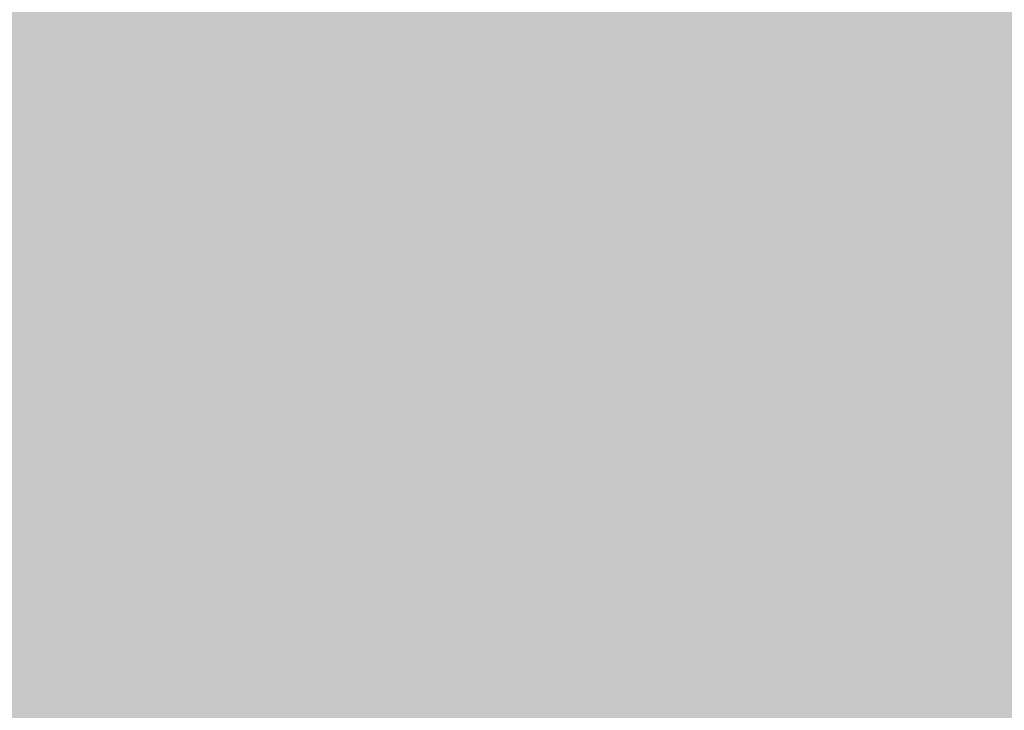
# Model space of a CAD drawing. Units: inches. Extents: x 2091 to 2899, y 967 to 2217.
# Tile 189 of 256: x 2203.16122 to 2203.18039, y 1152.26051 to 1152.27396. Entities that reach past the tile are written whole.
import ezdxf

# ---------------------------------------------------------------- set-up
doc = ezdxf.new("R2010")
doc.units = ezdxf.units.IN
doc.layers.add('A-WALL-PATT', color=141, linetype='Continuous', lineweight=13, true_color=0xadddf7)

msp = doc.modelspace()

# ---------------------------------------------------------------- hatches: boundary and pattern name
at = {"layer": 'A-WALL-PATT'}
h = msp.add_hatch(color=256, dxfattribs=at)
h.dxf.hatch_style = 1
h.paths.add_polyline_path([(2803.143603, 2050.919059), (2203.143603, 2050.919059), (2203.143603, 1090.919059), (2803.143603, 1090.919059)])
h.paths.add_polyline_path([(2635.79885, 1147.540465), (2674.524052, 1147.540465, 0.376086), (2678.529665, 1152.880202), (2678.529665, 1159.556473, 0.333335), (2674.524319, 1163.561846), (2674.524319, 1163.56185), (2674.524319, 1192.93439), (2635.805971, 1192.93439), (2597.087622, 1192.93439), (2597.087622, 1163.561846, 0.333335), (2593.082276, 1159.556473), (2593.082276, 1152.880202, 0.376086), (2597.087889, 1147.540465)], flags=0)
h.paths.add_polyline_path([(2436.010433, 1278.240778, 0.000483), (2435.952643, 1278.215027, -0.001328), (2435.935625, 1278.111693, -0.001711), (2436.11644, 1278.040758, 0.002185)], flags=0)
h.paths.add_polyline_path([(2794.143603, 1143.419059), (2794.143603, 1347.419059), (2543.370171, 1347.419059), (2543.370171, 1351.919059), (2794.143603, 1351.919059), (2794.143603, 1392.713555), (2793.947398, 1392.713555), (2793.947398, 1473.5369), (2794.143603, 1473.5369), (2794.143603, 1531.919059), (2650.143603, 1531.919059), (2650.143603, 1536.419059), (2794.143603, 1536.419059), (2794.143603, 1692.419059), (2609.375609, 1692.419059), (2609.375609, 1644.419059), (2604.875609, 1644.419059), (2604.875609, 1744.919059), (2609.375609, 1744.919059), (2609.375609, 1696.919059), (2794.143603, 1696.919059), (2794.143603, 1780.919059), (2609.643603, 1780.919059), (2493.875609, 1780.919059), (2493.875609, 1785.419059), (2609.643603, 1785.419059), (2794.143603, 1785.419059), (2794.143603, 1847.938821), (2793.951222, 1847.938821), (2793.951222, 1928.762166), (2794.143603, 1928.762166), (2794.143603, 1941.419059), (2614.143603, 1941.419059), (2614.143603, 1821.419059), (2609.643603, 1821.419059), (2609.643603, 1941.419059), (2392.143603, 1941.419059), (2392.143603, 1819.919059), (2387.643603, 1819.919059), (2387.643603, 1941.419059), (2212.143603, 1941.419059), (2212.143603, 1783.919059), (2392.143603, 1783.919059), (2392.143603, 1780.919059), (2212.143603, 1780.919059), (2212.143603, 1629.419059), (2387.643603, 1629.419059), (2387.643603, 1744.919059), (2392.143603, 1744.919059), (2392.143603, 1627.919059), (2317.143603, 1627.919059), (2317.143603, 1551.419059), (2317.143603, 1536.419059), (2459.383591, 1536.419059), (2459.383591, 1602.39648), (2463.883591, 1602.39648), (2463.883591, 1531.919059), (2456.643603, 1531.919059), (2456.643603, 1529.919059), (2452.143603, 1529.919059), (2452.143603, 1531.919059), (2312.643603, 1531.919059), (2312.643603, 1551.419059), (2306.143603, 1551.419059), (2306.143603, 1555.919059), (2308.143603, 1555.919059), (2308.143603, 1551.419059), (2312.643603, 1551.419059), (2312.643603, 1627.919059), (2212.143603, 1627.919059), (2212.143603, 1555.919059), (2270.143603, 1555.919059), (2270.143603, 1551.419059), (2212.143603, 1551.419059), (2212.143603, 1351.919059), (2272.143603, 1351.919059), (2272.143603, 1347.419059), (2212.143603, 1347.419059), (2212.143603, 1275.419059), (2308.143603, 1275.419059), (2308.143603, 1351.919059), (2452.143603, 1351.919059), (2452.143603, 1493.919059), (2456.643603, 1493.919059), (2456.643603, 1347.419059), (2312.643603, 1347.419059), (2312.643603, 1270.919059), (2212.143603, 1270.919059), (2212.143603, 1099.919059), (2281.237523, 1099.919059), (2282.871041, 1110.913803), (2282.008341, 1116.996603), (2278.557741, 1121.420403), (2268.205641, 1128.056203), (2272.087641, 1128.056203), (2273.812941, 1131.927003), (2279.420341, 1134.691903), (2285.027841, 1135.244903), (2287.615841, 1137.456803), (2288.047141, 1138.009803), (2289.341141, 1140.774703), (2291.066541, 1139.668703), (2292.360541, 1135.244903), (2295.379841, 1136.903803), (2296.242541, 1135.797903), (2297.105241, 1133.033003), (2300.124641, 1138.009803), (2303.143941, 1138.009803), (2304.437941, 1135.797903), (2303.143941, 1133.586003), (2306.594641, 1134.691903), (2307.888741, 1133.033003), (2310.908041, 1135.244903), (2313.927441, 1134.138903), (2315.62686, 1132.427102), (2308.320041, 1117.549603), (2290.203841, 1109.807903), (2288.909841, 1103.172103), (2289.272309, 1099.919059), (2434.918227, 1099.919059), (2431.593227, 1124.788059), (2429.930227, 1169.553059), (2430.927185, 1240.519694), (2435.658926, 1238.186126), (2437.135227, 1196.554059), (2438.798227, 1143.973059), (2442.678227, 1111.998059), (2446.558227, 1099.919059), (2794.143603, 1099.919059), (2794.143603, 1138.919059), (2548.032447, 1138.919059), (2548.032447, 1143.419059), (2548.032447, 1148.819059), (2546.668457, 1148.031559), (2528.685692, 1179.178622, 0.256256), (2512.032447, 1148.819059), (2512.032447, 1143.419059), (2512.032447, 1138.919059), (2507.532447, 1138.919059), (2507.532447, 1143.419059), (2507.532447, 1148.819059, 0.256256), (2490.879202, 1179.178622), (2472.896437, 1148.031559), (2471.532447, 1148.819059), (2471.532447, 1143.419059), (2467.032447, 1143.419059), (2467.032447, 1269.945786, 0.039061), (2460.909987, 1273.580059), (2467.032447, 1273.580059), (2467.032447, 1286.325364, 0.014511), (2465.216194, 1286.761905), (2467.032447, 1287.052576), (2467.032447, 1323.419059), (2471.532447, 1323.419059), (2471.532447, 1148.819059), (2489.532447, 1179.995973), (2490.896437, 1179.208473), (2490.879202, 1179.178622, -0.256256), (2507.532447, 1148.819059), (2507.532447, 1143.419059), (2512.032447, 1143.419059), (2512.032447, 1148.819059, -0.256256), (2528.685692, 1179.178622), (2528.668457, 1179.208473), (2530.032447, 1179.995973), (2548.032447, 1148.819059), (2548.032447, 1143.419059)], flags=16)
h.paths.add_polyline_path([(2607.768546, 1200.945083), (2607.768546, 1265.030625), (2597.087622, 1281.052011), (2619.784585, 1281.052011), (2627.795278, 1337.12686), (2635.79885, 1337.12686), (2643.816663, 1337.12686), (2651.827356, 1281.052011), (2674.524319, 1281.052011), (2663.843395, 1265.030625), (2663.843395, 1200.945083), (2635.805971, 1200.945083)], flags=0)
edge = h.paths.add_edge_path(flags=0)
edge.add_ellipse((13303.896215, 1272.998725), major_axis=(-10595.31304, 0.000001), ratio=0.842303870086, start_angle=0.6282372191, end_angle=0.6465540999, ccw=False)
edge.add_ellipse((2711.70045, 1156.852678), major_axis=(2.219769, 0), ratio=0.84230387, start_angle=111.535244, end_angle=180.628237, ccw=False)
edge.add_ellipse((13303.156292, 1272.998725), major_axis=(-10593.026306, 0), ratio=0.842303869544, start_angle=0.5282714718, end_angle=0.6465540971, ccw=False)
edge.add_line((2710.764596, 1175.333295), (2710.129986, 1175.333295))
edge.add_ellipse((2710.129986, 1176.579775), major_axis=(1.479846, 0), ratio=0.84230387, start_angle=180, end_angle=270, ccw=False)
edge.add_line((2708.65014, 1176.579775), (2708.65014, 1200.782914))
edge.add_ellipse((2710.129986, 1200.782914), major_axis=(1.479846, 0), ratio=0.84230387, start_angle=90, end_angle=180, ccw=False)
edge.add_line((2710.129986, 1202.029394), (2710.465075, 1202.029394))
edge.add_ellipse((13303.156292, 1272.998725), major_axis=(-10593.026306, 0), ratio=0.842303869544, start_angle=-0.0902290886, end_angle=0.3838667788, ccw=False)
edge.add_ellipse((2710.129986, 1290.927031), major_axis=(-1.479846, 0), ratio=0.84230387, start_angle=0, end_angle=90, ccw=False)
edge.add_line((2708.65014, 1290.927031), (2708.65014, 1315.13017))
edge.add_ellipse((2710.129986, 1315.13017), major_axis=(-1.479846, 0), ratio=0.84230387, start_angle=-90, end_angle=0, ccw=False)
edge.add_line((2710.129986, 1316.37665), (2710.706314, 1316.37665))
edge.add_ellipse((3238.40172, 1296.289566), major_axis=(528.234, 0), ratio=0.8423038695, start_angle=176.34957241, end_angle=177.82004969, ccw=False)
edge.add_ellipse((2775.063043, 1071.450696), major_axis=(313.307761, 0), ratio=0.8423038695, start_angle=102.12596555, end_angle=103.78052899, ccw=False)
edge.add_ellipse((2775.063043, 1078.305698), major_axis=(-305.302891, 0), ratio=0.8423038695, start_angle=-79.790461, end_angle=-77.55537271, ccw=False)
edge.add_ellipse((2695.141767, 1541.975383), major_axis=(-250.960216, 0), ratio=0.8423038695, start_angle=99.25656601, end_angle=102.55493264)
edge.add_line((2741.410326, 1334.214255), (2747.132545, 1337.378477))
edge.add_ellipse((2747.538616, 1336.857478), major_axis=(-0.739923, 0), ratio=0.8423039, start_angle=270, end_angle=307.93313, ccw=False)
edge.add_ellipse((2747.538616, 1336.857478), major_axis=(-0.739923, 0), ratio=0.8423039, start_angle=232.06687, end_angle=270, ccw=False)
edge.add_line((2747.944687, 1337.378477), (2753.666906, 1334.214255))
edge.add_ellipse((2799.935466, 1541.975383), major_axis=(250.960216, 0), ratio=0.8423038695, start_angle=257.44506736, end_angle=260.74343399)
edge.add_ellipse((2720.014189, 1078.305698), major_axis=(305.302891, 0), ratio=0.8423038695, start_angle=77.55537271, end_angle=79.790461, ccw=False)
edge.add_ellipse((2720.014189, 1071.450696), major_axis=(-313.307761, 0), ratio=0.8423038695, start_angle=256.21947101, end_angle=257.87403445, ccw=False)
edge.add_ellipse((2256.675512, 1296.289566), major_axis=(-528.234, 0), ratio=0.8423038695, start_angle=182.17995031, end_angle=183.65042759, ccw=False)
edge.add_line((2784.370918, 1316.37665), (2784.947247, 1316.37665))
edge.add_ellipse((2784.947247, 1315.13017), major_axis=(1.479846, 0), ratio=0.84230387, start_angle=0, end_angle=90, ccw=False)
edge.add_line((2786.427093, 1315.13017), (2786.427093, 1290.927031))
edge.add_ellipse((2784.947247, 1290.927031), major_axis=(1.479846, 0), ratio=0.84230387, start_angle=270, end_angle=360, ccw=False)
edge.add_ellipse((-7808.07906, 1272.998725), major_axis=(10593.026306, 0), ratio=0.842303869544, start_angle=-0.3838667788, end_angle=0.0902290886, ccw=False)
edge.add_line((2784.612157, 1202.029394), (2784.947247, 1202.029394))
edge.add_ellipse((2784.947247, 1200.782914), major_axis=(1.479846, 0), ratio=0.84230387, start_angle=0, end_angle=90, ccw=False)
edge.add_line((2786.427093, 1200.782914), (2786.427093, 1176.579775))
edge.add_ellipse((2784.947247, 1176.579775), major_axis=(-1.479846, 0), ratio=0.84230387, start_angle=90, end_angle=180, ccw=False)
edge.add_line((2784.947247, 1175.333295), (2784.312636, 1175.333295))
edge.add_ellipse((-7808.07906, 1272.998725), major_axis=(10593.026306, 0), ratio=0.842303869544, start_angle=-0.6186431963, end_angle=-0.5282714718, ccw=False)
edge.add_ellipse((2783.376783, 1156.852678), major_axis=(-2.219769, 0), ratio=0.84230387, start_angle=179.371763, end_angle=248.464757, ccw=False)
edge.add_ellipse((-7808.818983, 1272.998725), major_axis=(-10595.31304, 0.000004), ratio=0.842303865762, start_angle=179.3534459226, end_angle=179.3717628034, ccw=False)
edge.add_ellipse((2780.297303, 1153.500793), major_axis=(-5.246426, 0), ratio=0.84230387, start_angle=90, end_angle=179.353446, ccw=False)
edge.add_line((2780.297303, 1149.081708), (2714.77993, 1149.081708))
edge.add_ellipse((2714.77993, 1153.500793), major_axis=(5.246426, 0), ratio=0.84230387, start_angle=180.646554, end_angle=270, ccw=False)
edge = h.paths.add_edge_path(flags=0)
edge.add_line((2718.187367, 1151.007833), (2718.187367, 1170.472364))
edge.add_ellipse((2721.14706, 1170.472364), major_axis=(-2.959692, 0), ratio=0.84230387, start_angle=-90, end_angle=0, ccw=False)
edge.add_line((2721.14706, 1172.965324), (2773.930173, 1172.965324))
edge.add_ellipse((2773.930173, 1170.472364), major_axis=(-2.959692, 0), ratio=0.84230387, start_angle=180, end_angle=270, ccw=False)
edge.add_line((2776.889865, 1170.472364), (2776.889865, 1151.007833))
edge.add_line((2776.889865, 1151.007833), (2718.187367, 1151.007833))
edge = h.paths.add_edge_path(flags=0)
edge.add_line((2718.187367, 1180.23415), (2718.187367, 1199.057834))
edge.add_ellipse((2747.538616, 1320.39864), major_axis=(147.017924, 0), ratio=0.8423038695, start_angle=256.40186531, end_angle=283.59813469)
edge.add_line((2776.889865, 1199.057834), (2776.889865, 1180.23415))
edge.add_ellipse((2747.538616, 1301.574956), major_axis=(147.017924, 0), ratio=0.8423038695, start_angle=256.40186531, end_angle=283.59813469, ccw=False)
edge = h.paths.add_edge_path(flags=0)
edge.add_ellipse((13303.156292, 1272.998725), major_axis=(-10591.54646, 0), ratio=0.842303869555, start_angle=0.0555943135, end_angle=0.3777641939, ccw=False)
edge.add_line((2711.616859, 1262.72171), (2715.667408, 1249.495396))
edge.add_ellipse((6413.891963, 1241.691919), major_axis=(-3698.236159, 0), ratio=0.84230386955, start_angle=-0.120897369, end_angle=0.364076349)
edge.add_line((2715.761038, 1218.192455), (2711.934307, 1203.167361))
edge = h.paths.add_edge_path(flags=0)
edge.add_line((2718.187367, 1251.074566), (2716.002485, 1267.450435))
edge.add_ellipse((2742.151175, 1202.18954), major_axis=(81.772585, 0), ratio=0.84230387, start_angle=94.27742096, end_angle=111.8349538, ccw=False)
edge.add_line((2737.009748, 1270.930626), (2758.067484, 1270.930626))
edge.add_ellipse((2752.926058, 1202.18954), major_axis=(81.772585, 0), ratio=0.84230387, start_angle=68.1650462, end_angle=85.72257904, ccw=False)
edge.add_line((2779.074747, 1267.450435), (2776.889865, 1251.074566))
edge.add_ellipse((2750.338059, 1187.885356), major_axis=(79.579664, 0), ratio=0.84230387, start_angle=67.20808512, end_angle=85.1299304)
edge.add_line((2756.034656, 1254.743656), (2739.042576, 1254.743656))
edge.add_ellipse((2744.739174, 1187.885356), major_axis=(79.579664, 0), ratio=0.84230387, start_angle=94.8700696, end_angle=112.79191488)
edge = h.paths.add_edge_path(flags=0)
edge.add_line((2783.142926, 1203.167361), (2779.316194, 1218.192455))
edge.add_ellipse((-918.81473, 1241.691919), major_axis=(3698.236159, 0), ratio=0.84230386955, start_angle=-0.364076349, end_angle=0.120897369)
edge.add_line((2779.409825, 1249.495396), (2783.460373, 1262.72171))
edge.add_ellipse((-7808.07906, 1272.998725), major_axis=(-10591.54646, 0), ratio=0.84230386954, start_angle=179.6222358061, end_angle=179.9444056865, ccw=False)
edge = h.paths.add_edge_path(flags=0)
edge.add_ellipse((2734.200892, 1286.69044), major_axis=(-0.356609, 6.340078), ratio=0.60383358, start_angle=89.0020143, end_angle=253.657408, ccw=False)
edge.add_line((2730.369001, 1286.541806), (2730.369001, 1301.35198))
edge.add_line((2730.369001, 1301.35198), (2735.913311, 1305.214803))
edge.add_ellipse((2736.384917, 1304.734561), major_axis=(0.739923, 0), ratio=0.8423039, start_angle=90, end_angle=134.480211, ccw=False)
edge.add_line((2736.384917, 1305.357801), (2738.032783, 1305.357801))
edge.add_line((2738.032783, 1305.357801), (2738.032783, 1307.707927))
edge.add_ellipse((2794.201642, 1307.707927), major_axis=(56.168859, 0), ratio=0.84230387, start_angle=150.5614304, end_angle=180, ccw=False)
edge.add_ellipse((2700.875591, 1307.707927), major_axis=(-56.168859, 0), ratio=0.84230387, start_angle=180, end_angle=209.4385696, ccw=False)
edge.add_line((2757.04445, 1307.707927), (2757.04445, 1305.357801))
edge.add_line((2757.04445, 1305.357801), (2758.692316, 1305.357801))
edge.add_ellipse((2758.692316, 1304.734561), major_axis=(-0.739923, 0), ratio=0.8423039, start_angle=225.519789, end_angle=270, ccw=False)
edge.add_line((2759.163922, 1305.214803), (2764.708231, 1301.35198))
edge.add_line((2764.708231, 1301.35198), (2764.708231, 1286.541806))
edge.add_ellipse((2760.87634, 1286.69044), major_axis=(0.356609, 6.340078), ratio=0.60383358, start_angle=106.342592, end_angle=270.9979857, ccw=False)
edge.add_line((2757.04445, 1285.79709), (2757.04445, 1307.707927))
edge.add_ellipse((2700.875591, 1307.707927), major_axis=(-56.168859, 0), ratio=0.84230387, start_angle=180, end_angle=209.4385696)
edge.add_ellipse((2794.201642, 1307.707927), major_axis=(56.168859, 0), ratio=0.84230387, start_angle=150.5614304, end_angle=180)
edge.add_line((2738.032783, 1307.707927), (2738.032783, 1285.79709))
h.paths.add_polyline_path([(2417.812273, 1104.449704), (2413.492273, 1102.529704), (2410.612273, 1103.969704), (2409.172273, 1106.369704), (2407.252273, 1107.329704), (2406.292273, 1109.729704), (2405.332273, 1114.049704), (2405.332273, 1117.889704), (2406.292273, 1120.129704), (2407.252273, 1119.809704), (2408.848322, 1118.327658), (2410.173945, 1119.42417), (2410.211273, 1120.405704), (2411.040731, 1121.419054), (2410.699273, 1119.858704), (2410.173945, 1119.42417), (2410.088452, 1117.176109), (2411.132836, 1116.206324), (2413.972273, 1119.329704), (2416.852273, 1120.769704), (2416.869721, 1120.798784), (2417.035071, 1119.405116), (2417.896213, 1118.143384), (2418.292273, 1118.369704), (2419.544447, 1120.039269), (2419.360915, 1118.387487), (2419.032108, 1119.356151), (2418.398939, 1118.511926), (2419.252273, 1114.529704), (2418.794091, 1107.198795)], flags=0)
h.paths.add_polyline_path([(2508.870171, 1347.419059), (2508.370171, 1347.419059), (2508.370171, 1351.919059), (2508.870171, 1351.919059)], flags=0)
h.paths.add_polyline_path([(2473.370171, 1347.419059), (2472.370171, 1347.419059), (2467.870171, 1347.419059), (2467.870171, 1455.419059), (2472.370171, 1455.419059), (2472.370171, 1352.419059), (2473.370171, 1352.419059)], flags=0)
h.paths.add_polyline_path([(2352.106244, 1217.446197), (2349.226244, 1218.886197), (2347.786244, 1221.286197), (2345.866244, 1222.246197), (2344.906244, 1224.646197), (2343.946244, 1228.966197), (2343.946244, 1232.806197), (2344.906244, 1235.046197), (2345.866244, 1234.726197), (2347.462293, 1233.244152), (2348.787916, 1234.340663), (2348.825244, 1235.322197), (2349.654702, 1236.335547), (2349.313244, 1234.775197), (2348.787916, 1234.340663), (2348.702423, 1232.092603), (2349.746807, 1231.122817), (2352.586244, 1234.246197), (2355.466244, 1235.686197), (2355.483692, 1235.715277), (2355.649043, 1234.321609), (2356.510185, 1233.059877), (2356.906244, 1233.286197), (2358.158418, 1234.955762), (2357.974887, 1233.30398), (2357.646079, 1234.272644), (2357.012911, 1233.428419), (2357.866244, 1229.446197), (2357.408062, 1222.115288), (2356.426244, 1219.366197)], flags=0)
h.paths.add_polyline_path([(2348.2968, 1112.22442), (2347.0138, 1112.31042), (2345.5298, 1114.12742), (2345.7318, 1115.85842), (2346.8118, 1116.98242), (2346.8118, 1114.64642), (2345.8668, 1114.21442), (2346.8798, 1114.30042)], flags=0)
h.paths.add_polyline_path([(2347.0138, 1110.92642), (2346.2718, 1110.49342), (2346.6098, 1111.18642)], flags=0)
h.paths.add_polyline_path([(2345.8668, 1118.19442), (2345.5298, 1117.32942), (2343.7078, 1118.02142), (2344.3828, 1118.62642)], flags=0)
h.paths.add_polyline_path([(2346.6768, 1109.28242), (2346.0698, 1108.07142), (2345.8668, 1110.06142)], flags=0)
h.paths.add_polyline_path([(2345.0568, 1119.75142), (2343.6398, 1119.75142), (2343.9778, 1121.13542)], flags=0)
h.paths.add_polyline_path([(2345.2598, 1116.55042), (2345.1248, 1115.85842), (2344.9218, 1115.68542), (2344.7198, 1116.37742)], flags=0)
h.paths.add_polyline_path([(2345.6648, 1112.31042), (2345.4618, 1111.53242), (2344.0448, 1111.96442), (2344.6518, 1112.57042)], flags=0)
h.paths.add_polyline_path([(2345.1918, 1113.34942), (2344.4498, 1113.86842), (2344.7198, 1114.38742)], flags=0)
h.paths.add_polyline_path([(2344.6518, 1116.80942), (2344.1798, 1115.68542), (2344.6518, 1115.33942), (2343.9098, 1114.90642), (2343.0328, 1115.94442), (2343.6398, 1116.46342)], flags=0)
h.paths.add_polyline_path([(2345.8668, 1106.68642), (2344.9898, 1105.56242), (2344.5168, 1106.60042)], flags=0)
h.paths.add_polyline_path([(2344.8548, 1110.06142), (2344.5168, 1109.28242), (2344.1128, 1109.71542)], flags=0)
h.paths.add_polyline_path([(2344.0448, 1113.52242), (2343.4378, 1113.08942), (2342.7628, 1113.95442)], flags=0)
h.paths.add_polyline_path([(2344.3148, 1111.01242), (2342.9648, 1110.32042), (2342.9648, 1111.09942)], flags=0)
h.paths.add_polyline_path([(2345.1248, 1104.69742), (2344.5848, 1103.74542), (2344.4498, 1104.26442)], flags=0)
h.paths.add_polyline_path([(2342.8298, 1121.22242), (2341.7498, 1120.53042), (2340.5358, 1121.04942), (2340.1308, 1121.82842), (2340.6708, 1122.95242), (2341.1428, 1121.82842), (2341.6148, 1122.00142)], flags=0)
h.paths.add_polyline_path([(2342.9648, 1119.75142), (2343.0328, 1118.45342), (2342.0878, 1118.02142), (2342.0198, 1119.49142)], flags=0)
h.paths.add_polyline_path([(2342.6948, 1116.89642), (2341.9528, 1116.63642), (2342.0198, 1117.32942)], flags=0)
h.paths.add_polyline_path([(2343.0328, 1112.22442), (2342.0198, 1111.79142), (2341.5478, 1112.22442), (2342.3578, 1113.34942)], flags=0)
h.paths.add_polyline_path([(2343.7748, 1104.43742), (2342.6278, 1102.88042), (2342.6948, 1104.61042), (2343.4378, 1105.12942)], flags=0)
h.paths.add_polyline_path([(2342.0198, 1115.07942), (2340.8058, 1115.51242), (2340.9408, 1116.37742)], flags=0)
h.paths.add_polyline_path([(2341.4808, 1120.09742), (2341.4808, 1119.40542), (2341.0758, 1119.57842), (2341.1428, 1120.09742)], flags=0)
h.paths.add_polyline_path([(2341.8178, 1114.47342), (2340.9408, 1113.08942), (2340.8058, 1114.56042)], flags=0)
h.paths.add_polyline_path([(2341.1428, 1118.54042), (2340.9408, 1116.98242), (2339.0508, 1117.67542), (2339.0508, 1118.62642)], flags=0)
h.paths.add_polyline_path([(2342.6948, 1101.66842), (2341.9528, 1101.84142), (2342.5598, 1102.36142)], flags=0)
h.paths.add_polyline_path([(2340.3328, 1119.66542), (2338.4438, 1119.57842), (2337.9038, 1120.35742), (2339.6578, 1120.61642)], flags=0)
h.paths.add_polyline_path([(2340.3328, 1115.33942), (2340.0628, 1113.69542), (2339.3878, 1115.33942)], flags=0)
h.paths.add_polyline_path([(2341.8178, 1103.83142), (2341.5478, 1102.88042), (2341.1428, 1103.65842)], flags=0)
h.paths.add_polyline_path([(2339.0508, 1122.86642), (2337.2958, 1121.82842), (2337.0938, 1123.12542), (2337.7688, 1123.81842)], flags=0)
h.paths.add_polyline_path([(2339.1178, 1121.74142), (2338.8478, 1121.22242), (2338.1738, 1121.04942), (2338.3758, 1121.56842)], flags=0)
h.paths.add_polyline_path([(2339.1858, 1119.31942), (2338.6458, 1118.71342), (2338.2408, 1118.10742), (2338.2408, 1118.88642)], flags=0)
h.paths.add_polyline_path([(2341.1428, 1101.92842), (2340.6028, 1101.23642), (2340.0628, 1101.84142), (2340.6028, 1102.36142)], flags=0)
h.paths.add_polyline_path([(2337.6338, 1117.76142), (2336.6208, 1118.28042), (2337.2958, 1118.97242)], flags=0)
h.paths.add_polyline_path([(2336.8238, 1119.57842), (2334.7988, 1118.97242), (2335.2038, 1120.35742), (2336.5538, 1120.87642)], flags=0)
h.paths.add_polyline_path([(2339.1178, 1100.45742), (2337.3638, 1100.54342), (2336.7558, 1101.23642)], flags=0)
h.paths.add_polyline_path([(2336.3508, 1122.43342), (2336.0138, 1121.91442), (2334.9338, 1122.43342), (2334.5288, 1123.47142), (2335.7438, 1122.77942)], flags=0)
h.paths.add_polyline_path([(2334.7318, 1120.87642), (2334.2588, 1120.35742), (2334.0568, 1120.78942), (2334.5968, 1121.30842)], flags=0)
h.paths.add_polyline_path([(2334.4618, 1122.17442), (2332.5718, 1121.30842), (2331.3568, 1122.17442), (2332.0998, 1122.86642)], flags=0)
h.paths.add_polyline_path([(2334.2588, 1118.54042), (2333.3818, 1118.45342), (2333.6518, 1119.31942)], flags=0)
h.paths.add_polyline_path([(2335.5418, 1102.27442), (2334.1918, 1102.62042), (2335.2718, 1103.31242)], flags=0)
h.paths.add_polyline_path([(2332.7068, 1119.66542), (2331.6948, 1120.44342), (2332.5048, 1120.78942)], flags=0)
h.paths.add_polyline_path([(2334.7318, 1101.14942), (2333.5168, 1101.58242), (2333.9888, 1101.75542)], flags=0)
h.paths.add_polyline_path([(2332.6398, 1116.63642), (2331.0868, 1116.29042), (2331.9648, 1118.19442)], flags=0)
h.paths.add_polyline_path([(2330.7498, 1121.56842), (2330.2768, 1120.27042), (2328.5228, 1119.31942), (2328.9948, 1121.04942)], flags=0)
h.paths.add_polyline_path([(2330.7498, 1118.62642), (2330.0078, 1117.50242), (2329.8728, 1118.02142)], flags=0)
h.paths.add_polyline_path([(2332.0998, 1102.36142), (2330.5468, 1102.01442), (2331.6948, 1102.96642)], flags=0)
h.paths.add_polyline_path([(2329.5348, 1113.60842), (2329.0628, 1112.31042), (2328.5898, 1113.34942)], flags=0)
h.paths.add_polyline_path([(2328.3878, 1117.84842), (2327.5098, 1116.55042), (2327.1728, 1117.76142)], flags=0)
h.paths.add_polyline_path([(2329.7378, 1106.51342), (2329.5348, 1105.30242), (2328.2528, 1106.08142)], flags=0)
h.paths.add_polyline_path([(2328.6578, 1114.38742), (2328.0498, 1114.12742), (2328.3198, 1114.90642)], flags=0)
h.paths.add_polyline_path([(2328.3198, 1112.22442), (2327.1058, 1112.13742), (2326.7008, 1112.65642)], flags=0)
h.paths.add_polyline_path([(2326.9028, 1115.25242), (2326.7008, 1114.12742), (2325.2158, 1113.60842), (2326.0928, 1115.33942)], flags=0)
h.paths.add_polyline_path([(2326.6328, 1108.33042), (2326.0928, 1107.37942), (2325.8908, 1108.50342), (2326.4978, 1109.10942)], flags=0)
h.paths.add_polyline_path([(2615.143603, 1531.919059), (2609.643603, 1531.919059), (2609.643603, 1620.419059), (2614.143603, 1620.419059), (2614.143603, 1536.419059), (2615.143603, 1536.419059)], flags=0)
h.paths.add_polyline_path([(2545.143603, 1563.419059), (2464.143603, 1563.419059), (2464.143603, 1632.419059), (2509.143603, 1632.419059), (2509.143603, 1627.919059), (2509.143603, 1603.919059), (2468.643603, 1603.919059), (2468.643603, 1567.919059), (2540.643603, 1567.919059), (2540.643603, 1591.919059), (2545.143603, 1591.919059)], flags=0)
h.paths.add_polyline_path([(2388.969048, 1549.985735), (2357.434181, 1549.985735), (2357.434181, 1623.360778), (2399.362777, 1623.360778), (2435.689465, 1623.360778), (2435.592547, 1602.559273), (2435.592547, 1602.39648), (2388.969048, 1602.39648)], flags=0)
h.paths.add_polyline_path([(2388.880628, 1555.809151), (2374.904429, 1555.809151), (2374.904429, 1600.571564), (2374.904429, 1615.457645), (2406.350877, 1615.457645), (2406.350877, 1618.939431), (2412.174293, 1615.457645), (2406.350877, 1611.97586), (2406.350877, 1615.457645), (2388.880628, 1615.457645)], flags=0)
h.paths.add_polyline_path([(2568.875609, 1644.419059), (2453.375609, 1644.419059), (2453.375609, 1785.419059), (2457.875609, 1785.419059), (2457.875609, 1648.919059), (2568.875609, 1648.919059)], flags=0)
h.paths.add_polyline_path([(2212.143603, 1945.919059), (2212.143603, 2041.919059), (2794.143603, 2041.919059), (2794.143603, 1945.919059)], flags=16)
h.paths.add_polyline_path([(2271.082728, 1964.317238), (2776.852968, 1964.317238), (2776.852968, 2037.169623), (2271.082728, 2037.169623)], flags=8)
h.paths.add_polyline_path([(2380.649285, 1536.824144), (2461.040809, 1536.824144), (2461.040809, 1554.652587), (2380.649285, 1554.652587)], flags=8)
h.paths.add_polyline_path([(2240.755709, 1609.725451), (2309.185829, 1609.725451), (2309.185829, 1617.698204), (2240.755709, 1617.698204)], flags=8)
h.paths.add_polyline_path([(2212.677255, 1313.504102), (2282.59152, 1313.504102), (2282.59152, 1322.745239), (2212.677255, 1322.745239)], flags=8)
h.paths.add_polyline_path([(2457.111976, 1114.778574), (2558.481581, 1114.778574), (2558.481581, 1142.219682), (2457.111976, 1142.219682)], flags=8)
h.paths.add_polyline_path([(2473.442337, 1273.010067), (2604.641226, 1273.010067), (2604.641226, 1318.346935), (2473.442337, 1318.346935)], flags=8)
h.paths.add_polyline_path([(2638.876302, 1626.977432), (2684.250367, 1627.976738), (2684.038483, 1637.597494), (2638.664417, 1636.598188)], flags=8)
h.paths.add_polyline_path([(2537.590554, 1453.793447), (2628.389547, 1453.793447), (2628.389547, 1475.344811), (2537.590554, 1475.344811)], flags=8)
h.paths.add_polyline_path([(2504.137638, 1714.632397), (2554.647187, 1714.632397), (2554.647187, 1730.237712), (2504.137638, 1730.237712)], flags=8)
h.paths.add_polyline_path([(2487.501181, 1575.651872), (2535.097121, 1575.651872), (2535.097121, 1598.377646), (2487.501181, 1598.377646)], flags=8)
h.paths.add_polyline_path([(2709.0994, 1735.710278), (2740.016601, 1735.710278), (2740.016601, 1749.937641), (2709.0994, 1749.937641)], flags=8)
h.paths.add_polyline_path([(2442.438424, 1792.171657), (2564.728835, 1792.171657), (2564.728835, 1842.000163), (2442.438424, 1842.000163)], flags=8)
h.paths.add_polyline_path([(2655.815801, 1809.644076), (2789.520142, 1806.693796), (2790.084977, 1832.291638), (2656.380635, 1835.241918)], flags=8)
h.paths.add_polyline_path([(2234.842697, 1797.720143), (2368.592851, 1794.768852), (2369.160718, 1820.504132), (2235.410564, 1823.455423)], flags=8)
h.paths.add_polyline_path([(2245.138466, 1644.006335), (2398.427733, 1640.6239), (2398.994842, 1666.32482), (2245.705575, 1669.707255)], flags=8)
h.paths.add_polyline_path([(2306.142847, 1431.168519), (2413.768314, 1428.793687), (2414.333148, 1454.391529), (2306.707682, 1456.76636)], flags=8)
h.paths.add_polyline_path([(2306.834582, 1458.233145), (2393.380484, 1456.323449), (2393.932808, 1481.354358), (2307.386907, 1483.264054)], flags=8)

doc.saveas('drawing.dxf')
